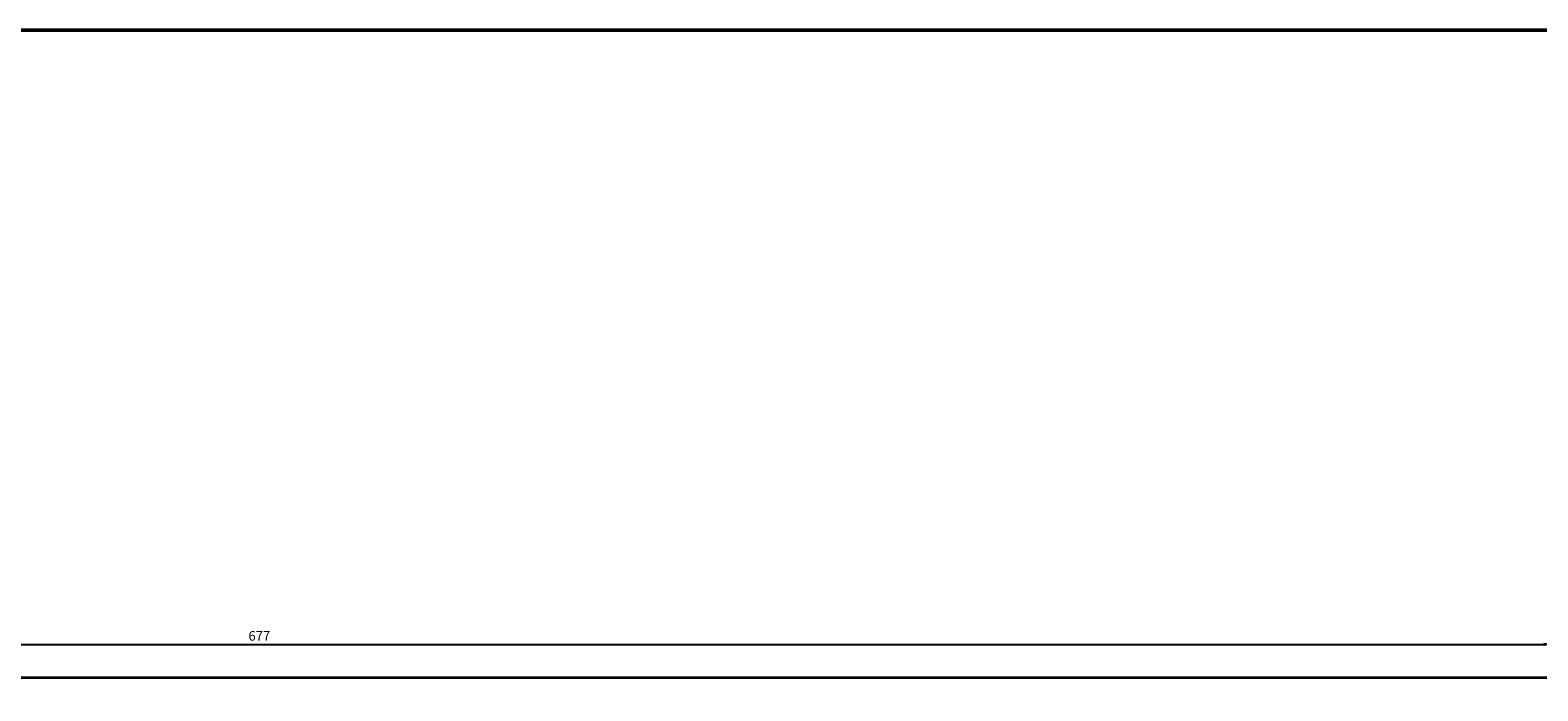
# Model space of a CAD drawing. Units: millimetres. Extents: x 2134 to 3363, y 1052 to 3233.
# Tile 10 of 11: x 2770 to 3165, y 3060 to 3233. Entities that reach past the tile are written whole.
import ezdxf

# ---------------------------------------------------------------- set-up
doc = ezdxf.new("R2010")
doc.units = ezdxf.units.MM
for name, color, linetype, lineweight in [('A-ANNO-DIMS', 2, 'Continuous', 18), ('A-ANNO-TTLB', 7, 'Continuous', 50), ('C-PROP', 6, 'Continuous', 35)]:
    doc.layers.add(name, color=color, linetype=linetype, lineweight=lineweight)
doc.styles.get("Standard").update_dxf_attribs({"font": 'arial.ttf'})
doc.dimstyles.new('ISO-25', dxfattribs={"dimtxt": 2.5, "dimasz": 2.5, "dimexe": 1.25, "dimexo": 0.625, "dimtad": 1, "dimtxsty": 'Standard', "dimcen": 2.5, "dimadec": 0, "dimazin": 0, "dimtfac": 1, "dimtmove": 0, "dimatfit": 3, "dimfxl": 1, "dimarcsym": 0})

# ---------------------------------------------------------------- blocks, each defined once
blk = doc.blocks.new('*D16')
at = {"layer": 'A-ANNO-DIMS', "color": 0, "lineweight": -2, "transparency": 16777216}
for p, q in [((2491.84, 3064.45), (2491.84, 3073.74)), ((3168.84, 3064.45), (3168.84, 3073.74)), ((2494.34, 3072.49), (3166.34, 3072.49))]:
    blk.add_line(p, q, dxfattribs=at)
at = {"layer": 'A-ANNO-DIMS', "color": 0, "transparency": 16777216}
for points in [[(2494.34, 3072.9), (2494.34, 3072.07), (2491.84, 3072.49)], [(3166.34, 3072.9), (3166.34, 3072.07), (3168.84, 3072.49)]]:
    blk.add_solid(points, dxfattribs=at)
at = {"layer": 'Defpoints', "color": 0, "transparency": 16777216}
for p in [(3168.84, 3072.49), (2491.84, 3063.82), (3168.84, 3063.82)]:
    blk.add_point(p, dxfattribs=at)
at = {"layer": 'A-ANNO-DIMS', "color": 0, "transparency": 16777216, "insert": (2830.34, 3074.39), "char_height": 2.5, "attachment_point": 5}
blk.add_mtext('677', dxfattribs=at)

msp = doc.modelspace()

# ---------------------------------------------------------------- linework, layer by layer
at = {"layer": 'A-ANNO-TTLB', "ltscale": 0.5}
msp.add_lwpolyline([(2134.34, 3233.23), (3362.77, 3233.23), (3362.77, 1152.237), (2134.34, 1152.237)], close=True, dxfattribs=at)
at = {"layer": 'C-PROP'}
msp.add_line((2491.839, 3063.82), (3168.839, 3063.82), dxfattribs=at)

# ---------------------------------------------------------------- dimensions: what is measured, and where the dimension line sits
at = {"layer": 'A-ANNO-DIMS'}
dim = msp.add_linear_dim(base=(3168.839, 3072.486), p1=(2491.839, 3063.82), p2=(3168.839, 3063.82), dimstyle='ISO-25', override={"dimclrd": 0, "dimclre": 0, "dimclrt": 0}, dxfattribs=at)
dim.commit()
dim.dimension.update_dxf_attribs({"geometry": '*D16', "text_midpoint": (2830.339, 3074.387)})

doc.saveas('drawing.dxf')
